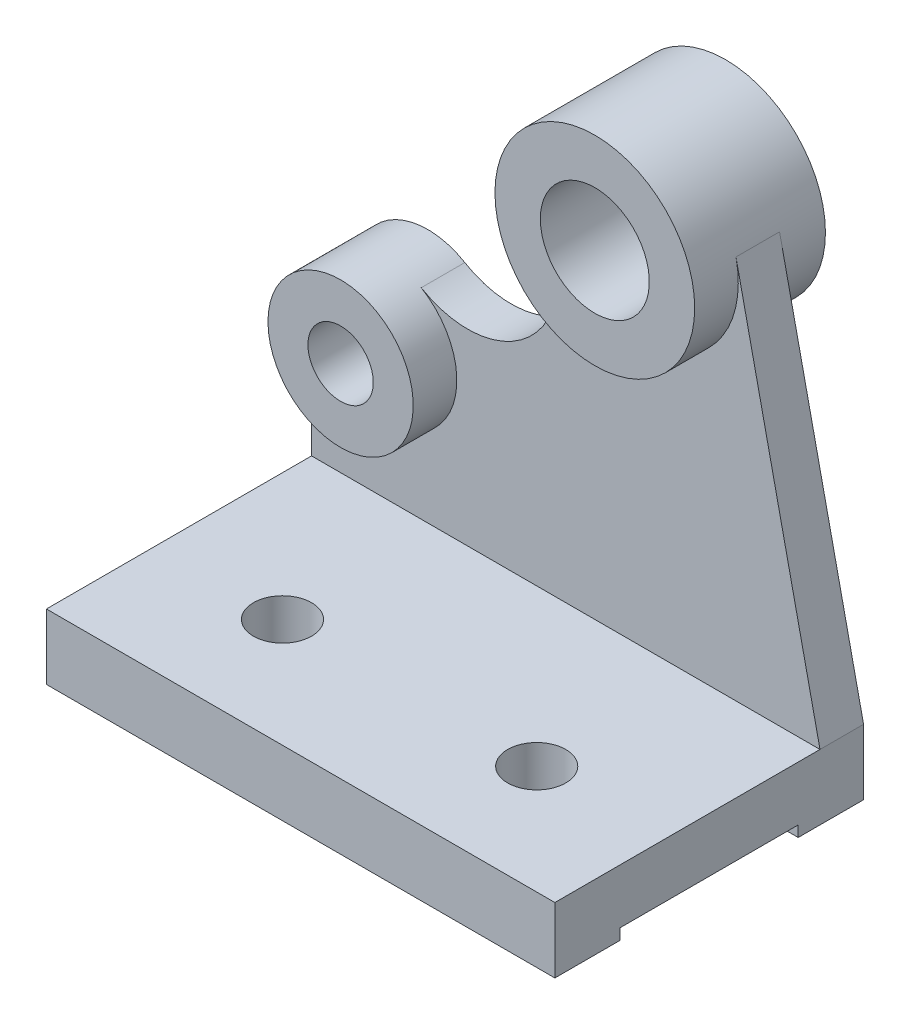
ISO-10303-21;
HEADER;
FILE_DESCRIPTION(('STEP AP214'),'2;1');
FILE_NAME('part.step','',(''),(''),'','','');
FILE_SCHEMA(('AUTOMOTIVE_DESIGN { 1 0 10303 214 1 1 1 1 }'));
ENDSEC;
DATA;
#1=APPLICATION_CONTEXT('core data for automotive mechanical design processes');
#2=APPLICATION_PROTOCOL_DEFINITION('international standard','automotive_design',2000,#1);
#3=PRODUCT_CONTEXT('',#1,'mechanical');
#4=PRODUCT('Part','Part','',(#3));
#5=PRODUCT_RELATED_PRODUCT_CATEGORY('part','',(#4));
#6=PRODUCT_DEFINITION_FORMATION('','',#4);
#7=PRODUCT_DEFINITION_CONTEXT('part definition',#1,'design');
#8=PRODUCT_DEFINITION('design','',#6,#7);
#9=PRODUCT_DEFINITION_SHAPE('','',#8);
#10=(LENGTH_UNIT() NAMED_UNIT(*) SI_UNIT(.MILLI.,.METRE.));
#11=(NAMED_UNIT(*) PLANE_ANGLE_UNIT() SI_UNIT($,.RADIAN.));
#12=(NAMED_UNIT(*) SI_UNIT($,.STERADIAN.) SOLID_ANGLE_UNIT());
#13=UNCERTAINTY_MEASURE_WITH_UNIT(LENGTH_MEASURE(1.E-05),#10,'distance_accuracy_value','');
#14=(GEOMETRIC_REPRESENTATION_CONTEXT(3) GLOBAL_UNCERTAINTY_ASSIGNED_CONTEXT((#13)) GLOBAL_UNIT_ASSIGNED_CONTEXT((#10,
#11,#12)) REPRESENTATION_CONTEXT('',''));
#15=CARTESIAN_POINT('',(0.,0.,0.));
#16=DIRECTION('',(0.,0.,1.));
#17=DIRECTION('',(1.,0.,0.));
#18=AXIS2_PLACEMENT_3D('',#15,#16,#17);
#19=CARTESIAN_POINT('',(0.,0.,0.));
#20=DIRECTION('',(0.,-1.,0.));
#21=DIRECTION('',(0.,0.,-1.));
#22=AXIS2_PLACEMENT_3D('',#19,#20,#21);
#23=PLANE('',#22);
#24=DIRECTION('',(1.,0.,0.));
#25=VECTOR('',#24,1.);
#26=CARTESIAN_POINT('',(-70.,0.,24.5));
#27=LINE('',#26,#25);
#28=CARTESIAN_POINT('',(-70.,0.,24.5));
#29=VERTEX_POINT('',#28);
#30=CARTESIAN_POINT('',(70.,0.,24.5));
#31=VERTEX_POINT('',#30);
#32=EDGE_CURVE('E192',#29,#31,#27,.T.);
#33=ORIENTED_EDGE('',*,*,#32,.T.);
#34=DIRECTION('',(0.,0.,-1.));
#35=VECTOR('',#34,1.);
#36=CARTESIAN_POINT('',(70.,0.,42.5));
#37=LINE('',#36,#35);
#38=CARTESIAN_POINT('',(70.,0.,42.5));
#39=VERTEX_POINT('',#38);
#40=EDGE_CURVE('E218',#39,#31,#37,.T.);
#41=ORIENTED_EDGE('',*,*,#40,.F.);
#42=DIRECTION('',(1.,0.,0.));
#43=VECTOR('',#42,1.);
#44=CARTESIAN_POINT('',(-70.,0.,42.5));
#45=LINE('',#44,#43);
#46=CARTESIAN_POINT('',(-70.,0.,42.5));
#47=VERTEX_POINT('',#46);
#48=EDGE_CURVE('E212',#47,#39,#45,.T.);
#49=ORIENTED_EDGE('',*,*,#48,.F.);
#50=DIRECTION('',(0.,0.,1.));
#51=VECTOR('',#50,1.);
#52=CARTESIAN_POINT('',(-70.,0.,42.5));
#53=LINE('',#52,#51);
#54=EDGE_CURVE('E221',#29,#47,#53,.T.);
#55=ORIENTED_EDGE('',*,*,#54,.F.);
#56=EDGE_LOOP('',(#33,#41,#49,#55));
#57=FACE_BOUND('',#56,.T.);
#58=ADVANCED_FACE('F39',(#57),#23,.T.);
#59=CARTESIAN_POINT('',(70.,18.,42.5));
#60=DIRECTION('',(-1.,0.,0.));
#61=DIRECTION('',(0.,0.,1.));
#62=AXIS2_PLACEMENT_3D('',#59,#60,#61);
#63=PLANE('',#62);
#64=ORIENTED_EDGE('',*,*,#40,.T.);
#65=DIRECTION('',(0.,-1.,0.));
#66=VECTOR('',#65,1.);
#67=CARTESIAN_POINT('',(70.,0.,24.5));
#68=LINE('',#67,#66);
#69=CARTESIAN_POINT('',(70.,3.,24.5));
#70=VERTEX_POINT('',#69);
#71=EDGE_CURVE('E193',#70,#31,#68,.T.);
#72=ORIENTED_EDGE('',*,*,#71,.F.);
#73=DIRECTION('',(0.,0.,1.));
#74=VECTOR('',#73,1.);
#75=CARTESIAN_POINT('',(70.,3.,24.5));
#76=LINE('',#75,#74);
#77=CARTESIAN_POINT('',(70.,3.,-24.5));
#78=VERTEX_POINT('',#77);
#79=EDGE_CURVE('E186',#78,#70,#76,.T.);
#80=ORIENTED_EDGE('',*,*,#79,.F.);
#81=DIRECTION('',(0.,1.,0.));
#82=VECTOR('',#81,1.);
#83=CARTESIAN_POINT('',(70.,0.,-24.5));
#84=LINE('',#83,#82);
#85=CARTESIAN_POINT('',(70.,0.,-24.5));
#86=VERTEX_POINT('',#85);
#87=EDGE_CURVE('E198',#86,#78,#84,.T.);
#88=ORIENTED_EDGE('',*,*,#87,.F.);
#89=CARTESIAN_POINT('',(70.,0.,-42.5));
#90=VERTEX_POINT('',#89);
#91=EDGE_CURVE('E201',#86,#90,#37,.T.);
#92=ORIENTED_EDGE('',*,*,#91,.T.);
#93=DIRECTION('',(0.,-1.,0.));
#94=VECTOR('',#93,1.);
#95=CARTESIAN_POINT('',(70.,18.,-42.5));
#96=LINE('',#95,#94);
#97=CARTESIAN_POINT('',(70.,18.,-42.5));
#98=VERTEX_POINT('',#97);
#99=EDGE_CURVE('E11',#98,#90,#96,.T.);
#100=ORIENTED_EDGE('',*,*,#99,.F.);
#101=DIRECTION('',(0.,0.,-1.));
#102=VECTOR('',#101,1.);
#103=CARTESIAN_POINT('',(70.,18.,-30.5));
#104=LINE('',#103,#102);
#105=CARTESIAN_POINT('',(70.,18.,-30.5));
#106=VERTEX_POINT('',#105);
#107=EDGE_CURVE('E173',#106,#98,#104,.T.);
#108=ORIENTED_EDGE('',*,*,#107,.F.);
#109=DIRECTION('',(0.,0.,-1.));
#110=VECTOR('',#109,1.);
#111=CARTESIAN_POINT('',(70.,18.,42.5));
#112=LINE('',#111,#110);
#113=CARTESIAN_POINT('',(70.,18.,42.5));
#114=VERTEX_POINT('',#113);
#115=EDGE_CURVE('E209',#114,#106,#112,.T.);
#116=ORIENTED_EDGE('',*,*,#115,.F.);
#117=DIRECTION('',(0.,-1.,0.));
#118=VECTOR('',#117,1.);
#119=CARTESIAN_POINT('',(70.,18.,42.5));
#120=LINE('',#119,#118);
#121=EDGE_CURVE('E217',#114,#39,#120,.T.);
#122=ORIENTED_EDGE('',*,*,#121,.T.);
#123=EDGE_LOOP('',(#64,#72,#80,#88,#92,#100,#108,#116,#122));
#124=FACE_BOUND('',#123,.T.);
#125=ADVANCED_FACE('F41',(#124),#63,.F.);
#126=CARTESIAN_POINT('',(-70.,18.,-42.5));
#127=DIRECTION('',(0.,0.,1.));
#128=DIRECTION('',(1.,0.,0.));
#129=AXIS2_PLACEMENT_3D('',#126,#127,#128);
#130=PLANE('',#129);
#131=DIRECTION('',(-1.,0.,0.));
#132=VECTOR('',#131,1.);
#133=CARTESIAN_POINT('',(-70.,0.,-42.5));
#134=LINE('',#133,#132);
#135=CARTESIAN_POINT('',(-70.,0.,-42.5));
#136=VERTEX_POINT('',#135);
#137=EDGE_CURVE('E225',#90,#136,#134,.T.);
#138=ORIENTED_EDGE('',*,*,#137,.T.);
#139=DIRECTION('',(0.,-1.,0.));
#140=VECTOR('',#139,1.);
#141=CARTESIAN_POINT('',(-70.,18.,-42.5));
#142=LINE('',#141,#140);
#143=CARTESIAN_POINT('',(-70.,56.,-42.5));
#144=VERTEX_POINT('',#143);
#145=EDGE_CURVE('E48',#144,#136,#142,.T.);
#146=ORIENTED_EDGE('',*,*,#145,.F.);
#147=CARTESIAN_POINT('',(-50.,56.,-42.5));
#148=DIRECTION('',(0.,0.,-1.));
#149=DIRECTION('',(-1.,0.,0.));
#150=AXIS2_PLACEMENT_3D('',#147,#148,#149);
#151=CIRCLE('',#150,20.);
#152=CARTESIAN_POINT('',(-39.8001548125971,73.2035798063372,-42.5));
#153=VERTEX_POINT('',#152);
#154=EDGE_CURVE('E292',#144,#153,#151,.T.);
#155=ORIENTED_EDGE('',*,*,#154,.T.);
#156=CARTESIAN_POINT('',(-27.0503483283434,94.7080545642588,-42.5));
#157=DIRECTION('',(0.,0.,1.));
#158=DIRECTION('',(-1.,0.,0.));
#159=AXIS2_PLACEMENT_3D('',#156,#157,#158);
#160=CIRCLE('',#159,25.);
#161=CARTESIAN_POINT('',(-4.64542055294179,105.799457152707,-42.5));
#162=VERTEX_POINT('',#161);
#163=EDGE_CURVE('E144',#153,#162,#160,.T.);
#164=ORIENTED_EDGE('',*,*,#163,.T.);
#165=CARTESIAN_POINT('',(20.,118.,-42.5));
#166=DIRECTION('',(0.,0.,1.));
#167=DIRECTION('',(-1.,0.,0.));
#168=AXIS2_PLACEMENT_3D('',#165,#166,#167);
#169=CIRCLE('',#168,27.5);
#170=CARTESIAN_POINT('',(46.8660884818626,123.870544240931,-42.5));
#171=VERTEX_POINT('',#170);
#172=EDGE_CURVE('E164',#162,#171,#169,.T.);
#173=ORIENTED_EDGE('',*,*,#172,.T.);
#174=DIRECTION('',(0.213474336033865,-0.97694867206773,0.));
#175=VECTOR('',#174,1.);
#176=CARTESIAN_POINT('',(70.,18.,-42.5));
#177=LINE('',#176,#175);
#178=EDGE_CURVE('E169',#171,#98,#177,.T.);
#179=ORIENTED_EDGE('',*,*,#178,.T.);
#180=ORIENTED_EDGE('',*,*,#99,.T.);
#181=EDGE_LOOP('',(#138,#146,#155,#164,#173,#179,#180));
#182=FACE_BOUND('',#181,.T.);
#183=CARTESIAN_POINT('',(-50.,56.,-42.5));
#184=DIRECTION('',(0.,0.,-1.));
#185=DIRECTION('',(-1.,0.,0.));
#186=AXIS2_PLACEMENT_3D('',#183,#184,#185);
#187=CIRCLE('',#186,9.);
#188=CARTESIAN_POINT('',(-59.,56.,-42.5));
#189=VERTEX_POINT('',#188);
#190=EDGE_CURVE('E330',#189,#189,#187,.T.);
#191=ORIENTED_EDGE('',*,*,#190,.F.);
#192=EDGE_LOOP('',(#191));
#193=FACE_BOUND('',#192,.T.);
#194=ADVANCED_FACE('F268',(#182,#193),#130,.F.);
#195=CARTESIAN_POINT('',(-70.,18.,42.5));
#196=DIRECTION('',(1.,0.,0.));
#197=DIRECTION('',(0.,0.,-1.));
#198=AXIS2_PLACEMENT_3D('',#195,#196,#197);
#199=PLANE('',#198);
#200=DIRECTION('',(0.,0.,1.));
#201=VECTOR('',#200,1.);
#202=CARTESIAN_POINT('',(-70.,3.,24.5));
#203=LINE('',#202,#201);
#204=CARTESIAN_POINT('',(-70.,3.,-24.5));
#205=VERTEX_POINT('',#204);
#206=CARTESIAN_POINT('',(-70.,3.,24.5));
#207=VERTEX_POINT('',#206);
#208=EDGE_CURVE('E187',#205,#207,#203,.T.);
#209=ORIENTED_EDGE('',*,*,#208,.T.);
#210=DIRECTION('',(0.,-1.,0.));
#211=VECTOR('',#210,1.);
#212=CARTESIAN_POINT('',(-70.,0.,24.5));
#213=LINE('',#212,#211);
#214=EDGE_CURVE('E183',#207,#29,#213,.T.);
#215=ORIENTED_EDGE('',*,*,#214,.T.);
#216=ORIENTED_EDGE('',*,*,#54,.T.);
#217=DIRECTION('',(0.,-1.,0.));
#218=VECTOR('',#217,1.);
#219=CARTESIAN_POINT('',(-70.,18.,42.5));
#220=LINE('',#219,#218);
#221=CARTESIAN_POINT('',(-70.,18.,42.5));
#222=VERTEX_POINT('',#221);
#223=EDGE_CURVE('E231',#222,#47,#220,.T.);
#224=ORIENTED_EDGE('',*,*,#223,.F.);
#225=DIRECTION('',(0.,0.,1.));
#226=VECTOR('',#225,1.);
#227=CARTESIAN_POINT('',(-70.,18.,42.5));
#228=LINE('',#227,#226);
#229=CARTESIAN_POINT('',(-70.,18.,-30.5));
#230=VERTEX_POINT('',#229);
#231=EDGE_CURVE('E213',#230,#222,#228,.T.);
#232=ORIENTED_EDGE('',*,*,#231,.F.);
#233=DIRECTION('',(0.,1.,0.));
#234=VECTOR('',#233,1.);
#235=CARTESIAN_POINT('',(-70.,18.,-30.5));
#236=LINE('',#235,#234);
#237=CARTESIAN_POINT('',(-70.,56.,-30.5));
#238=VERTEX_POINT('',#237);
#239=EDGE_CURVE('E57',#230,#238,#236,.T.);
#240=ORIENTED_EDGE('',*,*,#239,.T.);
#241=DIRECTION('',(0.,0.,-1.));
#242=VECTOR('',#241,1.);
#243=CARTESIAN_POINT('',(-70.,56.,-30.5));
#244=LINE('',#243,#242);
#245=EDGE_CURVE('E147',#238,#144,#244,.T.);
#246=ORIENTED_EDGE('',*,*,#245,.T.);
#247=ORIENTED_EDGE('',*,*,#145,.T.);
#248=CARTESIAN_POINT('',(-70.,0.,-24.5));
#249=VERTEX_POINT('',#248);
#250=EDGE_CURVE('E223',#136,#249,#53,.T.);
#251=ORIENTED_EDGE('',*,*,#250,.T.);
#252=DIRECTION('',(0.,1.,0.));
#253=VECTOR('',#252,1.);
#254=CARTESIAN_POINT('',(-70.,0.,-24.5));
#255=LINE('',#254,#253);
#256=EDGE_CURVE('E64',#249,#205,#255,.T.);
#257=ORIENTED_EDGE('',*,*,#256,.T.);
#258=EDGE_LOOP('',(#209,#215,#216,#224,#232,#240,#246,#247,#251,#257));
#259=FACE_BOUND('',#258,.T.);
#260=ADVANCED_FACE('F287',(#259),#199,.F.);
#261=CARTESIAN_POINT('',(-70.,18.,42.5));
#262=DIRECTION('',(0.,0.,-1.));
#263=DIRECTION('',(-1.,0.,0.));
#264=AXIS2_PLACEMENT_3D('',#261,#262,#263);
#265=PLANE('',#264);
#266=ORIENTED_EDGE('',*,*,#48,.T.);
#267=ORIENTED_EDGE('',*,*,#121,.F.);
#268=DIRECTION('',(1.,0.,0.));
#269=VECTOR('',#268,1.);
#270=CARTESIAN_POINT('',(-70.,18.,42.5));
#271=LINE('',#270,#269);
#272=EDGE_CURVE('E216',#222,#114,#271,.T.);
#273=ORIENTED_EDGE('',*,*,#272,.F.);
#274=ORIENTED_EDGE('',*,*,#223,.T.);
#275=EDGE_LOOP('',(#266,#267,#273,#274));
#276=FACE_BOUND('',#275,.T.);
#277=ADVANCED_FACE('F283',(#276),#265,.F.);
#278=CARTESIAN_POINT('',(0.,18.,0.));
#279=DIRECTION('',(0.,-1.,0.));
#280=DIRECTION('',(0.,0.,-1.));
#281=AXIS2_PLACEMENT_3D('',#278,#279,#280);
#282=PLANE('',#281);
#283=CARTESIAN_POINT('',(-35.,18.,12.5));
#284=DIRECTION('',(0.,1.,0.));
#285=DIRECTION('',(0.,0.,1.));
#286=AXIS2_PLACEMENT_3D('',#283,#284,#285);
#287=CIRCLE('',#286,8.);
#288=CARTESIAN_POINT('',(-35.,18.,20.5));
#289=VERTEX_POINT('',#288);
#290=EDGE_CURVE('E178',#289,#289,#287,.T.);
#291=ORIENTED_EDGE('',*,*,#290,.F.);
#292=EDGE_LOOP('',(#291));
#293=FACE_BOUND('',#292,.T.);
#294=CARTESIAN_POINT('',(35.,18.,12.5));
#295=DIRECTION('',(0.,1.,0.));
#296=DIRECTION('',(0.,0.,1.));
#297=AXIS2_PLACEMENT_3D('',#294,#295,#296);
#298=CIRCLE('',#297,8.);
#299=CARTESIAN_POINT('',(35.,18.,20.5));
#300=VERTEX_POINT('',#299);
#301=EDGE_CURVE('E171',#300,#300,#298,.T.);
#302=ORIENTED_EDGE('',*,*,#301,.F.);
#303=EDGE_LOOP('',(#302));
#304=FACE_BOUND('',#303,.T.);
#305=ORIENTED_EDGE('',*,*,#115,.T.);
#306=DIRECTION('',(-1.,0.,0.));
#307=VECTOR('',#306,1.);
#308=CARTESIAN_POINT('',(-70.,18.,-30.5));
#309=LINE('',#308,#307);
#310=EDGE_CURVE('E156',#106,#230,#309,.T.);
#311=ORIENTED_EDGE('',*,*,#310,.T.);
#312=ORIENTED_EDGE('',*,*,#231,.T.);
#313=ORIENTED_EDGE('',*,*,#272,.T.);
#314=EDGE_LOOP('',(#305,#311,#312,#313));
#315=FACE_BOUND('',#314,.T.);
#316=ADVANCED_FACE('F272',(#293,#304,#315),#282,.F.);
#317=DIRECTION('',(1.,0.,0.));
#318=VECTOR('',#317,1.);
#319=CARTESIAN_POINT('',(-70.,0.,-24.5));
#320=LINE('',#319,#318);
#321=EDGE_CURVE('E206',#249,#86,#320,.T.);
#322=ORIENTED_EDGE('',*,*,#321,.F.);
#323=ORIENTED_EDGE('',*,*,#250,.F.);
#324=ORIENTED_EDGE('',*,*,#137,.F.);
#325=ORIENTED_EDGE('',*,*,#91,.F.);
#326=EDGE_LOOP('',(#322,#323,#324,#325));
#327=FACE_BOUND('',#326,.T.);
#328=ADVANCED_FACE('F263',(#327),#23,.T.);
#329=CARTESIAN_POINT('',(-70.,0.,24.5));
#330=DIRECTION('',(0.,0.,1.));
#331=DIRECTION('',(1.,0.,0.));
#332=AXIS2_PLACEMENT_3D('',#329,#330,#331);
#333=PLANE('',#332);
#334=ORIENTED_EDGE('',*,*,#71,.T.);
#335=ORIENTED_EDGE('',*,*,#32,.F.);
#336=ORIENTED_EDGE('',*,*,#214,.F.);
#337=DIRECTION('',(1.,0.,0.));
#338=VECTOR('',#337,1.);
#339=CARTESIAN_POINT('',(-70.,3.,24.5));
#340=LINE('',#339,#338);
#341=EDGE_CURVE('E203',#207,#70,#340,.T.);
#342=ORIENTED_EDGE('',*,*,#341,.T.);
#343=EDGE_LOOP('',(#334,#335,#336,#342));
#344=FACE_BOUND('',#343,.T.);
#345=ADVANCED_FACE('F275',(#344),#333,.F.);
#346=CARTESIAN_POINT('',(-70.,3.,24.5));
#347=DIRECTION('',(0.,1.,0.));
#348=DIRECTION('',(0.,0.,1.));
#349=AXIS2_PLACEMENT_3D('',#346,#347,#348);
#350=PLANE('',#349);
#351=CARTESIAN_POINT('',(-35.,3.,12.5));
#352=DIRECTION('',(0.,1.,0.));
#353=DIRECTION('',(0.,0.,1.));
#354=AXIS2_PLACEMENT_3D('',#351,#352,#353);
#355=CIRCLE('',#354,8.);
#356=CARTESIAN_POINT('',(-35.,3.,20.5));
#357=VERTEX_POINT('',#356);
#358=EDGE_CURVE('E43',#357,#357,#355,.T.);
#359=ORIENTED_EDGE('',*,*,#358,.T.);
#360=EDGE_LOOP('',(#359));
#361=FACE_BOUND('',#360,.T.);
#362=CARTESIAN_POINT('',(35.,3.,12.5));
#363=DIRECTION('',(0.,1.,0.));
#364=DIRECTION('',(0.,0.,1.));
#365=AXIS2_PLACEMENT_3D('',#362,#363,#364);
#366=CIRCLE('',#365,8.);
#367=CARTESIAN_POINT('',(35.,3.,20.5));
#368=VERTEX_POINT('',#367);
#369=EDGE_CURVE('E185',#368,#368,#366,.T.);
#370=ORIENTED_EDGE('',*,*,#369,.T.);
#371=EDGE_LOOP('',(#370));
#372=FACE_BOUND('',#371,.T.);
#373=ORIENTED_EDGE('',*,*,#79,.T.);
#374=ORIENTED_EDGE('',*,*,#341,.F.);
#375=ORIENTED_EDGE('',*,*,#208,.F.);
#376=DIRECTION('',(1.,0.,0.));
#377=VECTOR('',#376,1.);
#378=CARTESIAN_POINT('',(-70.,3.,-24.5));
#379=LINE('',#378,#377);
#380=EDGE_CURVE('E204',#205,#78,#379,.T.);
#381=ORIENTED_EDGE('',*,*,#380,.T.);
#382=EDGE_LOOP('',(#373,#374,#375,#381));
#383=FACE_BOUND('',#382,.T.);
#384=ADVANCED_FACE('F243',(#361,#372,#383),#350,.F.);
#385=CARTESIAN_POINT('',(-70.,0.,-24.5));
#386=DIRECTION('',(0.,0.,-1.));
#387=DIRECTION('',(-1.,0.,0.));
#388=AXIS2_PLACEMENT_3D('',#385,#386,#387);
#389=PLANE('',#388);
#390=ORIENTED_EDGE('',*,*,#87,.T.);
#391=ORIENTED_EDGE('',*,*,#380,.F.);
#392=ORIENTED_EDGE('',*,*,#256,.F.);
#393=ORIENTED_EDGE('',*,*,#321,.T.);
#394=EDGE_LOOP('',(#390,#391,#392,#393));
#395=FACE_BOUND('',#394,.T.);
#396=ADVANCED_FACE('F258',(#395),#389,.F.);
#397=CARTESIAN_POINT('',(35.,0.,12.5));
#398=DIRECTION('',(0.,1.,0.));
#399=DIRECTION('',(0.,0.,1.));
#400=AXIS2_PLACEMENT_3D('',#397,#398,#399);
#401=CYLINDRICAL_SURFACE('',#400,8.);
#402=ORIENTED_EDGE('',*,*,#301,.T.);
#403=EDGE_LOOP('',(#402));
#404=FACE_BOUND('',#403,.T.);
#405=ORIENTED_EDGE('',*,*,#369,.F.);
#406=EDGE_LOOP('',(#405));
#407=FACE_BOUND('',#406,.T.);
#408=ADVANCED_FACE('F246',(#404,#407),#401,.F.);
#409=CARTESIAN_POINT('',(-35.,0.,12.5));
#410=DIRECTION('',(0.,1.,0.));
#411=DIRECTION('',(0.,0.,1.));
#412=AXIS2_PLACEMENT_3D('',#409,#410,#411);
#413=CYLINDRICAL_SURFACE('',#412,8.);
#414=ORIENTED_EDGE('',*,*,#290,.T.);
#415=EDGE_LOOP('',(#414));
#416=FACE_BOUND('',#415,.T.);
#417=ORIENTED_EDGE('',*,*,#358,.F.);
#418=EDGE_LOOP('',(#417));
#419=FACE_BOUND('',#418,.T.);
#420=ADVANCED_FACE('F241',(#416,#419),#413,.F.);
#421=CARTESIAN_POINT('',(70.,18.,-30.5));
#422=DIRECTION('',(0.97694867206773,0.213474336033865,0.));
#423=DIRECTION('',(-0.213474336033865,0.97694867206773,0.));
#424=AXIS2_PLACEMENT_3D('',#421,#422,#423);
#425=PLANE('',#424);
#426=ORIENTED_EDGE('',*,*,#178,.F.);
#427=DIRECTION('',(0.,0.,-1.));
#428=VECTOR('',#427,1.);
#429=CARTESIAN_POINT('',(46.8660884818626,123.870544240931,-30.5));
#430=LINE('',#429,#428);
#431=CARTESIAN_POINT('',(46.8660884818626,123.870544240931,-30.5));
#432=VERTEX_POINT('',#431);
#433=EDGE_CURVE('E174',#432,#171,#430,.T.);
#434=ORIENTED_EDGE('',*,*,#433,.F.);
#435=DIRECTION('',(0.213474336033865,-0.97694867206773,0.));
#436=VECTOR('',#435,1.);
#437=CARTESIAN_POINT('',(70.,18.,-30.5));
#438=LINE('',#437,#436);
#439=EDGE_CURVE('E161',#432,#106,#438,.T.);
#440=ORIENTED_EDGE('',*,*,#439,.T.);
#441=ORIENTED_EDGE('',*,*,#107,.T.);
#442=EDGE_LOOP('',(#426,#434,#440,#441));
#443=FACE_BOUND('',#442,.T.);
#444=ADVANCED_FACE('F242',(#443),#425,.T.);
#445=CARTESIAN_POINT('',(-27.0503483283434,94.7080545642588,-30.5));
#446=DIRECTION('',(0.,0.,-1.));
#447=DIRECTION('',(-1.,0.,0.));
#448=AXIS2_PLACEMENT_3D('',#445,#446,#447);
#449=CYLINDRICAL_SURFACE('',#448,25.);
#450=ORIENTED_EDGE('',*,*,#163,.F.);
#451=DIRECTION('',(0.,0.,-1.));
#452=VECTOR('',#451,1.);
#453=CARTESIAN_POINT('',(-39.8001548125971,73.2035798063372,-30.5));
#454=LINE('',#453,#452);
#455=CARTESIAN_POINT('',(-39.8001548125971,73.2035798063372,-30.5));
#456=VERTEX_POINT('',#455);
#457=EDGE_CURVE('E142',#456,#153,#454,.T.);
#458=ORIENTED_EDGE('',*,*,#457,.F.);
#459=CARTESIAN_POINT('',(-27.0503483283434,94.7080545642588,-30.5));
#460=DIRECTION('',(0.,0.,1.));
#461=DIRECTION('',(-1.,0.,0.));
#462=AXIS2_PLACEMENT_3D('',#459,#460,#461);
#463=CIRCLE('',#462,25.);
#464=CARTESIAN_POINT('',(-4.64542055294179,105.799457152707,-30.5));
#465=VERTEX_POINT('',#464);
#466=EDGE_CURVE('E133',#456,#465,#463,.T.);
#467=ORIENTED_EDGE('',*,*,#466,.T.);
#468=DIRECTION('',(0.,0.,-1.));
#469=VECTOR('',#468,1.);
#470=CARTESIAN_POINT('',(-4.64542055294179,105.799457152707,-30.5));
#471=LINE('',#470,#469);
#472=EDGE_CURVE('E149',#465,#162,#471,.T.);
#473=ORIENTED_EDGE('',*,*,#472,.T.);
#474=EDGE_LOOP('',(#450,#458,#467,#473));
#475=FACE_BOUND('',#474,.T.);
#476=ADVANCED_FACE('F141',(#475),#449,.F.);
#477=CARTESIAN_POINT('',(20.,118.,-30.5));
#478=DIRECTION('',(0.,0.,-1.));
#479=DIRECTION('',(-1.,0.,0.));
#480=AXIS2_PLACEMENT_3D('',#477,#478,#479);
#481=PLANE('',#480);
#482=ORIENTED_EDGE('',*,*,#310,.F.);
#483=ORIENTED_EDGE('',*,*,#439,.F.);
#484=CARTESIAN_POINT('',(20.,118.,-30.5));
#485=DIRECTION('',(0.,0.,1.));
#486=DIRECTION('',(-1.,0.,0.));
#487=AXIS2_PLACEMENT_3D('',#484,#485,#486);
#488=CIRCLE('',#487,27.5);
#489=EDGE_CURVE('E140',#465,#432,#488,.T.);
#490=ORIENTED_EDGE('',*,*,#489,.F.);
#491=ORIENTED_EDGE('',*,*,#466,.F.);
#492=CARTESIAN_POINT('',(-50.,56.,-30.5));
#493=DIRECTION('',(0.,0.,1.));
#494=DIRECTION('',(-1.,0.,0.));
#495=AXIS2_PLACEMENT_3D('',#492,#493,#494);
#496=CIRCLE('',#495,20.);
#497=EDGE_CURVE('E132',#238,#456,#496,.T.);
#498=ORIENTED_EDGE('',*,*,#497,.F.);
#499=ORIENTED_EDGE('',*,*,#239,.F.);
#500=EDGE_LOOP('',(#482,#483,#490,#491,#498,#499));
#501=FACE_BOUND('',#500,.T.);
#502=ADVANCED_FACE('F131',(#501),#481,.F.);
#503=CARTESIAN_POINT('',(20.,118.,-18.5));
#504=DIRECTION('',(0.,0.,-1.));
#505=DIRECTION('',(-1.,0.,0.));
#506=AXIS2_PLACEMENT_3D('',#503,#504,#505);
#507=CYLINDRICAL_SURFACE('',#506,27.5);
#508=CARTESIAN_POINT('',(20.,118.,-54.5));
#509=DIRECTION('',(0.,0.,-1.));
#510=DIRECTION('',(-1.,0.,0.));
#511=AXIS2_PLACEMENT_3D('',#508,#509,#510);
#512=CIRCLE('',#511,27.5);
#513=CARTESIAN_POINT('',(-7.49999999999997,118.,-54.5));
#514=VERTEX_POINT('',#513);
#515=EDGE_CURVE('E316',#514,#514,#512,.T.);
#516=ORIENTED_EDGE('',*,*,#515,.F.);
#517=EDGE_LOOP('',(#516));
#518=FACE_BOUND('',#517,.T.);
#519=CARTESIAN_POINT('',(20.,118.,-18.5));
#520=DIRECTION('',(0.,0.,-1.));
#521=DIRECTION('',(-1.,0.,0.));
#522=AXIS2_PLACEMENT_3D('',#519,#520,#521);
#523=CIRCLE('',#522,27.5);
#524=CARTESIAN_POINT('',(-7.49999999999997,118.,-18.5));
#525=VERTEX_POINT('',#524);
#526=EDGE_CURVE('E167',#525,#525,#523,.T.);
#527=ORIENTED_EDGE('',*,*,#526,.T.);
#528=EDGE_LOOP('',(#527));
#529=FACE_BOUND('',#528,.T.);
#530=ORIENTED_EDGE('',*,*,#172,.F.);
#531=ORIENTED_EDGE('',*,*,#472,.F.);
#532=ORIENTED_EDGE('',*,*,#489,.T.);
#533=ORIENTED_EDGE('',*,*,#433,.T.);
#534=EDGE_LOOP('',(#530,#531,#532,#533));
#535=FACE_BOUND('',#534,.T.);
#536=ADVANCED_FACE('F408',(#518,#529,#535),#507,.T.);
#537=CARTESIAN_POINT('',(20.,118.,-18.5));
#538=DIRECTION('',(0.,0.,-1.));
#539=DIRECTION('',(-1.,0.,0.));
#540=AXIS2_PLACEMENT_3D('',#537,#538,#539);
#541=PLANE('',#540);
#542=CARTESIAN_POINT('',(20.,118.,-18.5));
#543=DIRECTION('',(0.,0.,-1.));
#544=DIRECTION('',(-1.,0.,0.));
#545=AXIS2_PLACEMENT_3D('',#542,#543,#544);
#546=CIRCLE('',#545,15.);
#547=CARTESIAN_POINT('',(5.00000000000003,118.,-18.5));
#548=VERTEX_POINT('',#547);
#549=EDGE_CURVE('E311',#548,#548,#546,.T.);
#550=ORIENTED_EDGE('',*,*,#549,.T.);
#551=EDGE_LOOP('',(#550));
#552=FACE_BOUND('',#551,.T.);
#553=ORIENTED_EDGE('',*,*,#526,.F.);
#554=EDGE_LOOP('',(#553));
#555=FACE_BOUND('',#554,.T.);
#556=ADVANCED_FACE('F411',(#552,#555),#541,.F.);
#557=CARTESIAN_POINT('',(20.,118.,-18.5));
#558=DIRECTION('',(0.,0.,-1.));
#559=DIRECTION('',(-1.,0.,0.));
#560=AXIS2_PLACEMENT_3D('',#557,#558,#559);
#561=CYLINDRICAL_SURFACE('',#560,15.);
#562=ORIENTED_EDGE('',*,*,#549,.F.);
#563=EDGE_LOOP('',(#562));
#564=FACE_BOUND('',#563,.T.);
#565=CARTESIAN_POINT('',(20.,118.,-54.5));
#566=DIRECTION('',(0.,0.,-1.));
#567=DIRECTION('',(-1.,0.,0.));
#568=AXIS2_PLACEMENT_3D('',#565,#566,#567);
#569=CIRCLE('',#568,15.);
#570=CARTESIAN_POINT('',(5.00000000000003,118.,-54.5));
#571=VERTEX_POINT('',#570);
#572=EDGE_CURVE('E317',#571,#571,#569,.T.);
#573=ORIENTED_EDGE('',*,*,#572,.T.);
#574=EDGE_LOOP('',(#573));
#575=FACE_BOUND('',#574,.T.);
#576=ADVANCED_FACE('F425',(#564,#575),#561,.F.);
#577=CARTESIAN_POINT('',(20.,118.,-54.5));
#578=DIRECTION('',(0.,0.,-1.));
#579=DIRECTION('',(-1.,0.,0.));
#580=AXIS2_PLACEMENT_3D('',#577,#578,#579);
#581=PLANE('',#580);
#582=ORIENTED_EDGE('',*,*,#515,.T.);
#583=EDGE_LOOP('',(#582));
#584=FACE_BOUND('',#583,.T.);
#585=ORIENTED_EDGE('',*,*,#572,.F.);
#586=EDGE_LOOP('',(#585));
#587=FACE_BOUND('',#586,.T.);
#588=ADVANCED_FACE('F431',(#584,#587),#581,.T.);
#589=CARTESIAN_POINT('',(-50.,56.,-18.5));
#590=DIRECTION('',(0.,0.,-1.));
#591=DIRECTION('',(-1.,0.,0.));
#592=AXIS2_PLACEMENT_3D('',#589,#590,#591);
#593=CYLINDRICAL_SURFACE('',#592,20.);
#594=CARTESIAN_POINT('',(-50.,56.,-18.5));
#595=DIRECTION('',(0.,0.,-1.));
#596=DIRECTION('',(-1.,0.,0.));
#597=AXIS2_PLACEMENT_3D('',#594,#595,#596);
#598=CIRCLE('',#597,20.);
#599=CARTESIAN_POINT('',(-70.,56.,-18.5));
#600=VERTEX_POINT('',#599);
#601=EDGE_CURVE('E325',#600,#600,#598,.T.);
#602=ORIENTED_EDGE('',*,*,#601,.T.);
#603=EDGE_LOOP('',(#602));
#604=FACE_BOUND('',#603,.T.);
#605=ORIENTED_EDGE('',*,*,#245,.F.);
#606=ORIENTED_EDGE('',*,*,#497,.T.);
#607=ORIENTED_EDGE('',*,*,#457,.T.);
#608=ORIENTED_EDGE('',*,*,#154,.F.);
#609=EDGE_LOOP('',(#605,#606,#607,#608));
#610=FACE_BOUND('',#609,.T.);
#611=ADVANCED_FACE('F153',(#604,#610),#593,.T.);
#612=CARTESIAN_POINT('',(-50.,56.,-18.5));
#613=DIRECTION('',(0.,0.,-1.));
#614=DIRECTION('',(-1.,0.,0.));
#615=AXIS2_PLACEMENT_3D('',#612,#613,#614);
#616=PLANE('',#615);
#617=CARTESIAN_POINT('',(-50.,56.,-18.5));
#618=DIRECTION('',(0.,0.,-1.));
#619=DIRECTION('',(-1.,0.,0.));
#620=AXIS2_PLACEMENT_3D('',#617,#618,#619);
#621=CIRCLE('',#620,9.);
#622=CARTESIAN_POINT('',(-59.,56.,-18.5));
#623=VERTEX_POINT('',#622);
#624=EDGE_CURVE('E322',#623,#623,#621,.T.);
#625=ORIENTED_EDGE('',*,*,#624,.T.);
#626=EDGE_LOOP('',(#625));
#627=FACE_BOUND('',#626,.T.);
#628=ORIENTED_EDGE('',*,*,#601,.F.);
#629=EDGE_LOOP('',(#628));
#630=FACE_BOUND('',#629,.T.);
#631=ADVANCED_FACE('F334',(#627,#630),#616,.F.);
#632=CARTESIAN_POINT('',(-50.,56.,-18.5));
#633=DIRECTION('',(0.,0.,-1.));
#634=DIRECTION('',(-1.,0.,0.));
#635=AXIS2_PLACEMENT_3D('',#632,#633,#634);
#636=CYLINDRICAL_SURFACE('',#635,9.);
#637=ORIENTED_EDGE('',*,*,#624,.F.);
#638=EDGE_LOOP('',(#637));
#639=FACE_BOUND('',#638,.T.);
#640=ORIENTED_EDGE('',*,*,#190,.T.);
#641=EDGE_LOOP('',(#640));
#642=FACE_BOUND('',#641,.T.);
#643=ADVANCED_FACE('F338',(#639,#642),#636,.F.);
#644=CLOSED_SHELL('',(#58,#125,#194,#260,#277,#316,#328,#345,#384,#396,#408,#420,#444,#476,#502,
#536,#556,#576,#588,#611,#631,#643));
#645=MANIFOLD_SOLID_BREP('B2',#644);
#646=ADVANCED_BREP_SHAPE_REPRESENTATION('',(#18,#645),#14);
#647=SHAPE_DEFINITION_REPRESENTATION(#9,#646);
ENDSEC;
END-ISO-10303-21;
